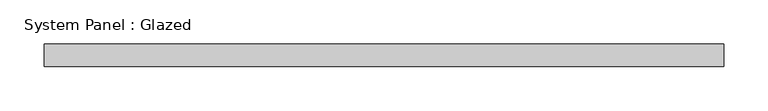
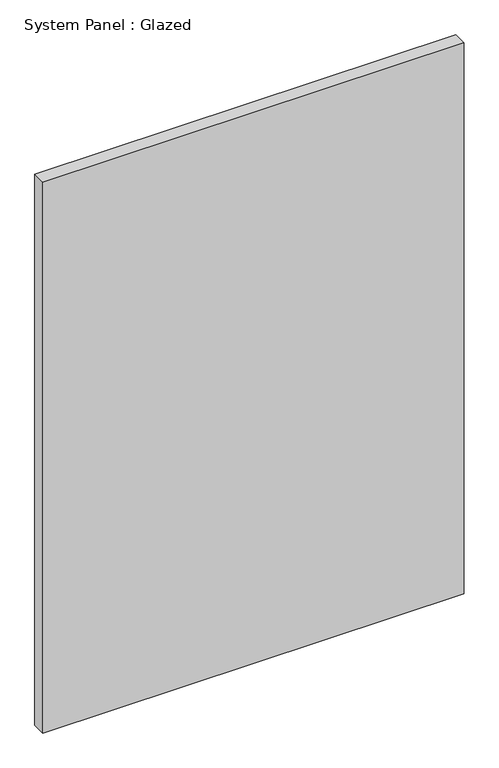
"""IFC4 building model written with IfcOpenShell, lengths in millimetres: plate geometry, System Panel : Glazed."""

from ifc_helpers import new_model, si_unit, origin, origin_with_axes, place, context, project, spatial, polyline, outline, extrude, source, transform, mapped, element, save


def system_panel_glazed_a35be92d(model_context):
    return source(origin(), model_context, "Body", "SweptSolid", [
        extrude(outline(polyline([(383.50825, 19.05), (-383.50825, 19.05), (-383.50825, 44.45), (383.50825, 44.45), (383.50825, 19.05)])), origin_with_axes(), (0.0, 0.0, 1.0), 1059.561),
    ])


if __name__ == "__main__":
    model = new_model("IFC4")
    model_context = context("Model", 3, world=origin())
    ifc_project = project(units=[si_unit("LENGTHUNIT", "METRE", prefix="MILLI")], contexts=[model_context])
    site = spatial("IfcSite", under=ifc_project)
    building = spatial("IfcBuilding", under=site)
    placement = place(None, origin())
    system_panel_glazed_shape = system_panel_glazed_a35be92d(model_context)
    element("IfcPlate", 1, ObjectType="System Panel : Glazed", at=placement, inside=building, context=model_context, shape_type="MappedRepresentation", body=[
        mapped(system_panel_glazed_shape, transform((0.0, 0.0, 0.0), x_axis=(1.0, 0.0, 0.0), y_axis=(0.0, 1.0, 0.0), z_axis=(0.0, 0.0, 1.0))),
    ])
    save(model, "model.ifc")

# Revit data of these elements
# Type "System Panel : Glazed"
#   Construction Type Id = "GSP4R"
#   Analytic Construction = "1/8 in Pilkington single glazing"
#   Visual Light Transmittance = 0.9
#   Solar Heat Gain Coefficient = 0.86
#   Heat Transfer Coefficient (U) = 1.18115 BTU/(h·ft²·°F)
#   Define Thermal Properties by = 1
# Element 1 (IfcPlate, "System Panel : Glazed")
#   Materials on its faces: "Glass"
# Materials
#   "Glass": class "Glass", colour RGB 0 128 192, transparency 0.75, Description = "Soda Lime Glass", Cost = 0
